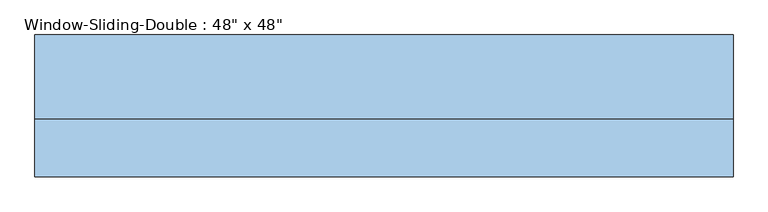
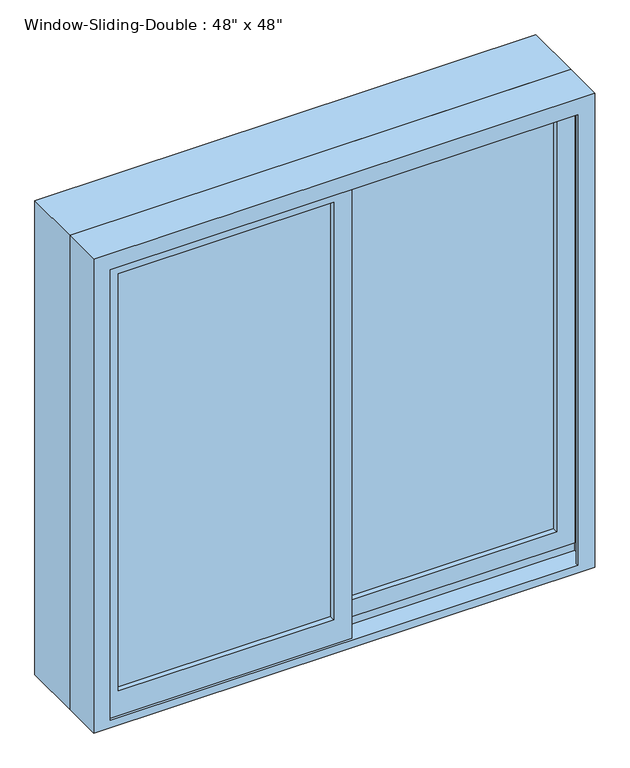
"""IFC4 building model written with IfcOpenShell, lengths in millimetres: window geometry."""

from ifc_helpers import new_model, si_unit, frame, origin, place, context, project, spatial, polyline, outline, extrude, faceted_brep, source, transform, mapped, element, save


def window_c1e3dfc0(model_context):
    return source(origin(), model_context, "Body", "SolidModel", [
        extrude(outline(polyline([(952.5, -22.225), (952.5, 590.55), (2114.55, 590.55), (2114.55, -22.225), (952.5, -22.225)]), holes=[polyline([(996.95, 546.1), (996.95, 22.225), (2070.1, 22.225), (2070.1, 546.1), (996.95, 546.1)])]), frame((0.0, -78.74, 0.0), z_axis=(0.0, 1.0, 0.0), x_axis=(0.0, 0.0, 1.0)), (0.0, 0.0, 1.0), 44.45),
        extrude(outline(polyline([(933.45, 22.225), (2114.55, 22.225), (2114.55, -590.55), (933.45, -590.55), (933.45, 22.225)]), holes=[polyline([(2070.1, -546.1), (2070.1, -22.225), (996.95, -22.225), (996.95, -546.1), (2070.1, -546.1)])]), frame((0.0, -123.19, 0.0), z_axis=(0.0, 1.0, 0.0), x_axis=(0.0, 0.0, 1.0)), (0.0, 0.0, 1.0), 44.45),
        extrude(outline(polyline([(-22.225, -110.49), (-546.1, -110.49), (-546.1, -104.14), (-22.225, -104.14), (-22.225, -110.49)])), frame((0.0, 0.0, 996.95), z_axis=(0.0, 0.0, 1.0), x_axis=(1.0, 0.0, 0.0)), (0.0, 0.0, 1.0), 1073.15),
        extrude(outline(polyline([(-22.225, -97.79), (-546.1, -97.79), (-546.1, -91.44), (-22.225, -91.44), (-22.225, -97.79)])), frame((0.0, 0.0, 996.95), z_axis=(0.0, 0.0, 1.0), x_axis=(1.0, 0.0, 0.0)), (0.0, 0.0, 1.0), 1073.15),
        extrude(outline(polyline([(546.1, -66.04), (22.225, -66.04), (22.225, -59.69), (546.1, -59.69), (546.1, -66.04)])), frame((0.0, 0.0, 996.95), z_axis=(0.0, 0.0, 1.0), x_axis=(1.0, 0.0, 0.0)), (0.0, 0.0, 1.0), 1073.15),
        extrude(outline(polyline([(546.1, -53.34), (22.225, -53.34), (22.225, -46.99), (546.1, -46.99), (546.1, -53.34)])), frame((0.0, 0.0, 996.95), z_axis=(0.0, 0.0, 1.0), x_axis=(1.0, 0.0, 0.0)), (0.0, 0.0, 1.0), 1073.15),
        extrude(outline(polyline([(2133.6, 609.6), (2133.6, -609.6), (914.4, -609.6), (914.4, 609.6), (2133.6, 609.6)]), holes=[polyline([(2114.55, -590.55), (2114.55, 590.55), (933.45, 590.55), (933.45, -590.55), (2114.55, -590.55)])]), frame((0.0, -27.94, 0.0), z_axis=(0.0, 1.0, 0.0), x_axis=(0.0, 0.0, 1.0)), (0.0, 0.0, 1.0), 146.05),
        faceted_brep([(-609.6, -27.94, 914.4), (609.6, -27.94, 914.4), (609.6, -129.54, 914.4), (-609.6, -129.54, 914.4), (-568.6778905, -129.54, 2092.6778905), (-568.6778905, -129.54, 933.45), (-568.6778905, -123.19, 933.45), (-568.6778905, -123.19, 2092.6778905), (-590.55, -123.19, 933.45), (-590.55, -123.19, 2114.55), (590.55, -123.19, 2114.55), (590.55, -123.19, 933.45), (568.6778905, -123.19, 933.45), (568.6778905, -123.19, 2092.6778905), (-590.55, -78.74, 933.45), (-590.55, -78.74, 952.5), (-590.55, -34.29, 952.5), (-590.55, -34.29, 933.45), (-590.55, -27.94, 933.45), (-590.55, -27.94, 2114.55), (-609.6, -27.94, 2133.6), (609.6, -27.94, 2133.6), (590.55, -27.94, 2114.55), (590.55, -27.94, 933.45), (-609.6, -129.54, 2133.6), (609.6, -129.54, 2133.6), (568.6778905, -129.54, 2092.6778905), (568.6778905, -129.54, 933.45), (590.55, -34.29, 933.45), (590.55, -34.29, 952.5), (590.55, -78.74, 952.5), (590.55, -78.74, 933.45)], [[[0, 1, 2, 3]], [[4, 5, 6, 7]], [[7, 6, 8, 9, 10, 11, 12, 13]], [[9, 8, 14, 15, 16, 17, 18, 19]], [[0, 20, 21, 1], [22, 19, 18, 23]], [[24, 20, 0, 3]], [[2, 25, 24, 3], [4, 26, 27, 5]], [[7, 13, 26, 4]], [[9, 19, 22, 10]], [[20, 24, 25, 21]], [[13, 12, 27, 26]], [[22, 23, 28, 29, 30, 31, 11, 10]], [[21, 25, 2, 1]], [[27, 12, 11, 31, 14, 8, 6, 5]], [[31, 30, 15, 14]], [[30, 29, 16, 15]], [[29, 28, 17, 16]], [[18, 17, 28, 23]]]),
    ])


if __name__ == "__main__":
    model = new_model("IFC4")
    model_context = context("Model", 3, world=origin())
    ifc_project = project(units=[si_unit("LENGTHUNIT", "METRE", prefix="MILLI")], contexts=[model_context])
    site = spatial("IfcSite", under=ifc_project)
    building = spatial("IfcBuilding", under=site)
    placement = place(None, origin())
    window_shape = window_c1e3dfc0(model_context)
    element("IfcWindow", 1, ObjectType="Window-Sliding-Double : 48\" x 48\"", at=placement, inside=building, context=model_context, shape_type="MappedRepresentation", body=[
        mapped(window_shape, transform((0.0, 0.0, 0.0), x_axis=(1.0, 0.0, 0.0), y_axis=(0.0, 1.0, 0.0), z_axis=(0.0, 0.0, 1.0))),
    ])
    save(model, "model.ifc")

# Revit data of these elements
# Type "Window-Sliding-Double : 48\" x 48\""
#   Type Mark = "23"
#   Fire Rating = "0.5h"
#   Assembly Code = "B2020100"
#   Analytic Construction = "Double glazing - domestic"
#   Window Inset [instance default] = 0' - 0"
#   Wall Thickness [instance default] = 0' - 6"
#   Visual Light Transmittance = 0.81
#   Thermal Resistance (R) = 1.8146 (h·ft²·°F)/BTU
#   Solar Heat Gain Coefficient = 0.76
#   Muntin Width = 1' - 8 5/8"
#   Muntin Height = 3' - 6 1/4"
#   Interior Wall Closure [instance default] = 0' - 2 3/4"
#   Heat Transfer Coefficient (U) = 0.5511 BTU/(h·ft²·°F)
#   Frame Extension [instance default] = 0' - 0 1/4"
#   Exterior Wall Closure [instance default] = 0' - 1 1/4"
#   Rough Width = 4' - 0 1/2"
#   Rough Height = 4' - 0 1/2"
#   Height = 4' - 0"
#   Extension Jamb [instance default] = 0' - 2 3/4"
#   Default Sill Height = 3' - 0"
#   Width = 4' - 0"
#   Interior Trim Visibility [instance default] = yes
#   Indicator Visibility [instance default] = yes
#   Exterior Trim Visibility [instance default] = yes
#   Muntin Visibility = yes
#   Extension Jamb Visibility [instance default] = yes
#   Muntin Pattern = Muntin Pattern_2x2 : Muntin Pattern_2x2
#   Interior Trim Material = Wood - Stained
#   Interior Trim = Trim-Window-Interior-Flat : Picture Frame
#   Interior Frame Material = Wood - Stained
#   Glass Panel Material = Glass
#   Exterior Trim Material = Clad - White
#   Exterior Trim = Trim-Window-Exterior-Flat : with Sill
#   Exterior Frame Material = Clad - White
#   Wall Closure = (empty or 0)
# Element 1 (IfcWindow, "Window-Sliding-Double : 48\" x 48\"")
#   Wall Thickness = 0' - 9"
#   Extension Jamb = 0' - 5 3/4"
#   Materials on its faces: "Wood - Stained", "Glass", "Clad - White"
# Materials
#   "Wood - Stained": class "Wood", colour RGB 224 178 126, transparency 0, Cost = 0
#   "Glass": class "Glass", colour RGB 0 128 192, transparency 0.75, Description = "Soda Lime Glass", Cost = 0
#   "Clad - White": class "Wood", colour RGB 242 242 238, transparency 0, Cost = 0
